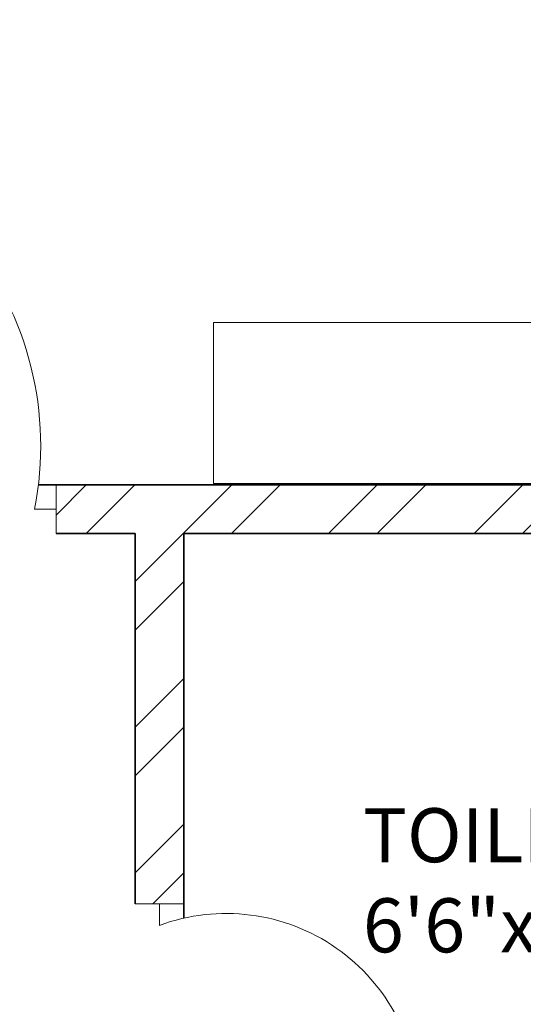
# Model space of a CAD drawing. Units: inches. Extents: x 2168 to 3056, y 1130 to 2629.
# Tile 35 of 42: x 2771 to 2818, y 2217 to 2308. Entities that reach past the tile are written whole.
import ezdxf

# ---------------------------------------------------------------- set-up
doc = ezdxf.new("R2010")
doc.units = ezdxf.units.IN
for name, color, linetype, lineweight in [('A-AREA-IDEN', 7, 'Continuous', 18), ('A-DOOR', 21, 'Continuous', 18), ('A-FLOR-CASE', 71, 'Continuous', 18), ('A-WALL', 7, 'Continuous', 35)]:
    doc.layers.add(name, color=color, linetype=linetype, lineweight=lineweight)
doc.layers.add('A-WALL-PATT', color=143, linetype='Continuous', lineweight=13, true_color=0x7aafdf)
doc.styles.get("Standard").update_dxf_attribs({"font": 'arial.ttf'})

# ---------------------------------------------------------------- blocks, each defined once
blk = doc.blocks.new('CUPBOARD-BEDROOM')
blk.add_lwpolyline([(0, 14.894), (70.359, 14.894), (70.359, 0), (0, 0)], close=True)

msp = doc.modelspace()

# ---------------------------------------------------------------- hatches: boundary and pattern name
at = {"layer": 'A-WALL-PATT'}
h = msp.add_hatch(dxfattribs=at)
h.set_pattern_fill('ANSI32', color=256)
h.paths.add_polyline_path([(2463.796, 2409.389), (2467.387, 2409.389), (2467.387, 2413.889), (2454.768, 2413.889), (2454.768, 2411.639), (2454.768, 2409.389), (2459.296, 2409.389), (2459.296, 2265.389), (2455.644, 2265.389), (2455.644, 2260.889), (2467.349, 2260.889), (2467.349, 2263.139), (2467.349, 2265.389), (2463.796, 2265.389)])
h.paths.add_polyline_path([(2431.596, 2413.889), (2409.647, 2413.889), (2409.647, 2409.389), (2431.596, 2409.389), (2431.596, 2411.639)])
h.paths.add_polyline_path([(2349.647, 2413.889), (2331.796, 2413.889), (2331.796, 2362.671), (2336.296, 2362.671), (2336.296, 2409.389), (2349.647, 2409.389), (2349.647, 2411.639)])
h.paths.add_polyline_path([(2634.149, 2411.639), (2634.149, 2413.889), (2562.293, 2413.889), (2562.293, 2409.389), (2595.796, 2409.389), (2595.796, 2280.309), (2595.826, 2280.309), (2595.826, 2265.389), (2499.91, 2265.389), (2499.91, 2260.889), (2550.796, 2260.889), (2550.796, 2117.308), (2555.296, 2117.308), (2555.296, 2168.08), (2571.93, 2168.08), (2571.93, 2176.889), (2559.796, 2176.889), (2559.796, 2256.389), (2640.796, 2256.389), (2640.796, 2176.889), (2626.428, 2176.889), (2626.428, 2168.08), (2645.296, 2168.08), (2645.296, 2116.637), (2649.796, 2116.637), (2649.796, 2260.889), (2691.251, 2260.889), (2691.251, 2263.139), (2691.251, 2265.389), (2670.655, 2265.389), (2670.655, 2265.365), (2600.296, 2265.365), (2600.296, 2280.258), (2600.296, 2409.389), (2634.149, 2409.389)])
h.paths.add_polyline_path([(2600.296, 2473.889), (2612.84, 2473.889), (2612.84, 2478.389), (2572.636, 2478.389), (2572.636, 2473.889), (2595.796, 2473.889), (2595.796, 2413.889), (2600.296, 2413.889)])
h.paths.add_polyline_path([(2535.796, 2473.889), (2548.636, 2473.889), (2548.636, 2478.389), (2531.396, 2478.389), (2531.396, 2413.889), (2521.6, 2413.889), (2521.6, 2409.389), (2539.239, 2409.389), (2539.239, 2411.639), (2539.239, 2413.889), (2535.796, 2413.889)])
h.paths.add_polyline_path([(2664.796, 2478.389), (2636.84, 2478.389), (2636.84, 2473.889), (2660.296, 2473.889), (2660.296, 2413.889), (2656.165, 2413.889), (2656.165, 2409.389), (2671.684, 2409.389), (2671.684, 2411.639), (2671.684, 2413.889), (2664.796, 2413.889)])
h.paths.add_polyline_path([(2705.942, 2413.889), (2695.684, 2413.889), (2695.684, 2409.389), (2705.942, 2409.389)])
h.paths.add_polyline_path([(2741.35, 2413.889), (2728.733, 2413.889), (2728.733, 2411.639), (2728.733, 2409.389), (2732.296, 2409.389), (2732.296, 2265.389), (2725.733, 2265.389), (2725.733, 2260.889), (2740.917, 2260.889), (2740.917, 2263.139), (2740.917, 2265.389), (2736.796, 2265.389), (2736.796, 2409.389), (2741.35, 2409.389)])
h.paths.add_polyline_path([(2785.655, 2413.889), (2764.546, 2413.889), (2764.486, 2409.389), (2785.655, 2409.389), (2785.655, 2411.639)])
h.paths.add_polyline_path([(2864.296, 2413.889), (2845.655, 2413.889), (2845.655, 2409.389), (2859.796, 2409.389), (2859.796, 2368.425), (2864.296, 2368.425)])
h.paths.add_polyline_path([(2864.296, 2308.425), (2862.046, 2308.425), (2859.796, 2308.425), (2859.796, 2265.389), (2774.483, 2265.389), (2774.483, 2263.139), (2774.483, 2260.889), (2781.796, 2260.889), (2781.796, 2226.654), (2786.296, 2226.654), (2786.296, 2260.889), (2859.796, 2260.889), (2859.796, 2241.352), (2864.296, 2241.352)])
h.paths.add_polyline_path([(2864.296, 2217.352), (2862.046, 2217.352), (2859.796, 2217.352), (2859.796, 2200.889), (2786.296, 2200.889), (2786.296, 2205.931), (2784.046, 2205.931), (2781.796, 2205.931), (2781.796, 2150.974), (2786.296, 2150.974), (2786.296, 2161.889), (2859.796, 2161.889), (2859.796, 2144.419), (2864.296, 2144.419)])
h.paths.add_polyline_path([(2859.796, 2196.389), (2859.796, 2166.389), (2786.296, 2166.389), (2786.296, 2196.389)], flags=16)
h.paths.add_polyline_path([(2864.296, 2108.419), (2862.046, 2108.419), (2859.796, 2108.419), (2859.796, 2080.889), (2786.296, 2080.889), (2786.296, 2111.993), (2781.796, 2111.993), (2781.796, 2080.889), (2649.796, 2080.889), (2649.796, 2086.036), (2647.546, 2086.036), (2645.296, 2086.036), (2645.296, 2071.739), (2649.796, 2071.739), (2649.796, 2076.389), (2781.796, 2076.389), (2781.796, 2041.792), (2786.296, 2041.792), (2786.296, 2076.389), (2859.796, 2076.389), (2859.796, 2058.577), (2864.296, 2058.577)])
h.paths.add_polyline_path([(2864.296, 2022.577), (2859.796, 2022.577), (2859.796, 1992.389), (2786.296, 1992.389), (2786.296, 1999.573), (2781.796, 1999.573), (2781.796, 1848.085), (2784.046, 1848.085), (2786.296, 1848.085), (2786.296, 1851.389), (2859.796, 1851.389), (2859.796, 1838.258), (2864.296, 1838.258)], flags=17)
h.paths.add_polyline_path([(2859.796, 1987.889), (2859.796, 1855.889), (2786.296, 1855.889), (2786.296, 1987.889)], flags=16)
h.paths.add_polyline_path([(2823.046, 1987.889), (2841.421, 1921.889), (2823.046, 1855.889)], flags=0)
h.paths.add_polyline_path([(2864.296, 1814.258), (2859.796, 1814.258), (2859.796, 1791.389), (2786.296, 1791.389), (2786.296, 1825.658), (2784.046, 1825.658), (2781.796, 1825.658), (2781.796, 1791.389), (2720.155, 1791.389), (2720.155, 1791.265), (2649.796, 1791.265), (2649.796, 1806.159), (2649.796, 2038.983), (2647.546, 2038.983), (2645.296, 2038.983), (2645.296, 1783.925), (2649.796, 1783.925), (2649.796, 1786.889), (2781.796, 1786.889), (2781.796, 1746.789), (2786.296, 1746.789), (2786.296, 1786.889), (2859.796, 1786.889), (2859.796, 1770.083), (2864.296, 1770.083)])
h.paths.add_polyline_path([(2864.296, 1734.083), (2862.046, 1734.083), (2859.796, 1734.083), (2859.796, 1705.889), (2786.296, 1705.889), (2786.296, 1714.166), (2781.796, 1714.166), (2781.796, 1660.527), (2786.296, 1660.527), (2786.296, 1666.889), (2859.796, 1666.889), (2859.796, 1648.342), (2864.296, 1648.342)])
h.paths.add_polyline_path([(2786.296, 1701.389), (2859.796, 1701.389), (2859.796, 1671.389), (2786.296, 1671.389)], flags=16)
h.paths.add_polyline_path([(2649.796, 1756.576), (2647.546, 1756.576), (2645.296, 1756.576), (2645.296, 1606.889), (2555.296, 1606.889), (2555.296, 1749.513), (2553.046, 1749.513), (2550.796, 1749.513), (2550.796, 1606.889), (2503.006, 1606.889), (2503.006, 1604.639), (2503.006, 1602.389), (2595.796, 1602.389), (2595.849, 1602.389), (2595.849, 1587.495), (2595.796, 1458.389), (2561.502, 1458.389), (2561.502, 1456.139), (2561.502, 1453.889), (2595.796, 1453.889), (2595.796, 1381.889), (2573.438, 1381.889), (2573.438, 1377.389), (2613.01, 1377.389), (2613.01, 1379.639), (2613.01, 1381.889), (2600.296, 1381.889), (2600.296, 1453.889), (2634.327, 1453.889), (2634.327, 1458.389), (2600.296, 1458.389), (2600.296, 1602.389), (2670.655, 1602.389), (2694.095, 1602.389), (2694.095, 1606.889), (2649.796, 1606.889)])
h.paths.add_polyline_path([(2736.796, 1602.389), (2741.562, 1602.389), (2741.562, 1606.889), (2726.203, 1606.889), (2726.203, 1604.639), (2726.203, 1602.389), (2732.296, 1602.389), (2732.296, 1458.389), (2727.899, 1458.389), (2727.899, 1453.889), (2740.821, 1453.889), (2740.821, 1456.139), (2740.821, 1458.389), (2736.796, 1458.389)])
h.paths.add_polyline_path([(2859.796, 1606.889), (2786.296, 1606.889), (2786.296, 1637.334), (2784.046, 1637.334), (2781.796, 1637.334), (2781.796, 1606.889), (2775.612, 1606.889), (2775.612, 1602.389), (2859.796, 1602.389)])
h.paths.add_polyline_path([(2864.296, 1624.342), (2862.046, 1624.342), (2859.796, 1624.342), (2859.796, 1570.39), (2864.296, 1570.39)])
h.paths.add_polyline_path([(2864.296, 1510.39), (2862.046, 1510.39), (2859.796, 1510.39), (2859.796, 1458.389), (2846.735, 1458.389), (2846.735, 1456.139), (2846.735, 1453.889), (2864.296, 1453.889)])
h.paths.add_polyline_path([(2786.735, 1458.389), (2765.444, 1458.389), (2765.444, 1453.889), (2786.735, 1453.889)])
h.paths.add_polyline_path([(2706.004, 1458.389), (2695.36, 1458.389), (2695.36, 1453.889), (2706.004, 1453.889), (2706.004, 1456.139)])
h.paths.add_polyline_path([(2671.36, 1456.139), (2671.36, 1458.389), (2655.986, 1458.389), (2655.986, 1456.139), (2655.986, 1453.889), (2660.296, 1453.889), (2660.296, 1381.889), (2637.01, 1381.889), (2637.01, 1377.389), (2664.796, 1377.389), (2664.796, 1453.889), (2671.36, 1453.889)], flags=17)
h.paths.add_polyline_path([(2539.829, 1458.389), (2520.237, 1458.389), (2520.237, 1453.889), (2531.296, 1453.889), (2531.296, 1377.389), (2546.449, 1377.389), (2546.449, 1379.639), (2546.449, 1381.889), (2535.796, 1381.889), (2535.796, 1453.889), (2539.829, 1453.889)], flags=17)
h.paths.add_polyline_path([(2496.237, 1458.389), (2489.13, 1458.389), (2489.13, 1453.889), (2496.237, 1453.889), (2496.237, 1456.139)])
h.paths.add_polyline_path([(2467.433, 1456.139), (2467.433, 1458.389), (2463.796, 1458.389), (2463.796, 1602.389), (2468.242, 1602.389), (2468.242, 1605.7), (2468.242, 1606.889), (2454.602, 1606.889), (2454.602, 1602.389), (2459.296, 1602.389), (2459.296, 1458.389), (2454.24, 1458.389), (2454.24, 1453.889), (2467.433, 1453.889)])
h.paths.add_polyline_path([(2431.601, 1456.139), (2431.601, 1458.389), (2411.386, 1458.389), (2411.386, 1453.889), (2431.601, 1453.889)])
h.paths.add_polyline_path([(2351.386, 1458.389), (2336.296, 1458.389), (2336.296, 1490.693), (2334.046, 1490.693), (2331.796, 1490.693), (2331.796, 1453.889), (2351.386, 1453.889), (2351.386, 1456.139)])
h.paths.add_polyline_path([(2336.296, 1629.705), (2331.796, 1629.705), (2331.796, 1552.317), (2336.296, 1552.317), (2336.296, 1602.389), (2406.655, 1602.389), (2423.472, 1602.389), (2423.472, 1606.889), (2418.796, 1606.889), (2418.796, 1643.678), (2416.546, 1643.678), (2414.296, 1643.678), (2414.296, 1606.889), (2336.296, 1606.889)])
h.paths.add_polyline_path([(2418.796, 1714.384), (2414.296, 1714.384), (2414.296, 1705.889), (2336.296, 1705.889), (2336.296, 1731.324), (2334.046, 1731.324), (2331.796, 1731.324), (2331.796, 1653.705), (2334.046, 1653.705), (2336.296, 1653.705), (2336.296, 1666.889), (2414.296, 1666.889), (2414.296, 1663.589), (2418.796, 1663.589)])
h.paths.add_polyline_path([(2336.296, 1701.389), (2414.296, 1701.389), (2414.296, 1671.389), (2336.296, 1671.389)], flags=16)
h.paths.add_polyline_path([(2555.296, 2040.059), (2550.796, 2040.059), (2550.796, 1791.389), (2550.561, 1791.205), (2480.202, 1791.205), (2418.796, 1791.389), (2418.796, 1825.448), (2416.546, 1825.448), (2414.296, 1825.448), (2414.296, 1791.389), (2336.296, 1791.389), (2336.296, 1806.409), (2331.796, 1806.409), (2331.796, 1767.324), (2336.296, 1767.324), (2336.296, 1786.889), (2414.296, 1786.889), (2414.296, 1745.457), (2418.796, 1745.457), (2418.796, 1786.889), (2550.796, 1786.889), (2550.796, 1783.011), (2555.296, 1783.011)])
h.paths.add_polyline_path([(2418.796, 1923.389), (2423.207, 1923.389), (2423.207, 1925.639), (2423.207, 1927.889), (2418.796, 1927.889), (2418.796, 2000.048), (2414.296, 2000.048), (2414.296, 1992.389), (2336.296, 1992.389), (2336.296, 1987.889), (2414.296, 1987.889), (2414.296, 1855.889), (2336.296, 1855.889), (2336.296, 1851.389), (2414.296, 1851.389), (2414.296, 1846.759), (2418.796, 1846.759)], flags=17)
h.paths.add_polyline_path([(2336.296, 2019.294), (2334.046, 2019.294), (2331.796, 2019.294), (2331.796, 1830.409), (2336.296, 1830.409)], flags=17)
h.paths.add_polyline_path([(2550.796, 1927.889), (2453.541, 1927.889), (2453.541, 1925.639), (2453.541, 1923.389), (2550.796, 1923.389)], flags=17)
h.paths.add_polyline_path([(2744.987, 1927.889), (2649.796, 1927.889), (2649.796, 1923.389), (2744.987, 1923.389), (2744.987, 1925.639)], flags=17)
h.paths.add_polyline_path([(2555.296, 2086.458), (2553.046, 2086.458), (2550.796, 2086.458), (2550.796, 2080.889), (2418.796, 2080.889), (2336.296, 2080.889), (2336.296, 2115.399), (2334.046, 2115.399), (2331.796, 2115.399), (2331.796, 2055.294), (2336.296, 2055.294), (2336.296, 2076.389), (2550.796, 2076.389), (2550.796, 2071.538), (2555.296, 2071.538)])
h.paths.add_polyline_path([(2418.796, 2121.389), (2414.296, 2121.389), (2414.296, 2080.889), (2418.796, 2080.889)])
h.paths.add_polyline_path([(2418.796, 2076.389), (2414.296, 2076.389), (2414.296, 2035.123), (2418.796, 2035.123)])
h.paths.add_polyline_path([(2422.868, 2263.139), (2422.868, 2265.389), (2406.655, 2265.389), (2406.655, 2265.359), (2336.296, 2265.359), (2336.296, 2280.252), (2336.296, 2302.671), (2334.046, 2302.671), (2331.796, 2302.671), (2331.796, 2246.853), (2336.296, 2246.853), (2336.296, 2260.889), (2414.296, 2260.889), (2414.296, 2223.996), (2418.796, 2223.996), (2418.796, 2260.889), (2422.868, 2260.889)])
h.paths.add_polyline_path([(2418.796, 2204.783), (2416.546, 2204.783), (2414.296, 2204.783), (2414.296, 2200.889), (2336.296, 2200.889), (2336.296, 2220.853), (2331.796, 2220.853), (2331.796, 2151.399), (2336.296, 2151.399), (2336.296, 2161.889), (2414.296, 2161.889), (2414.296, 2153.726), (2418.796, 2153.726)])
h.paths.add_polyline_path([(2414.296, 2196.389), (2414.296, 2166.389), (2336.296, 2166.389), (2336.296, 2196.389)], flags=16)
h.paths.add_polyline_path([(2375.296, 2181.389), (2336.296, 2166.389), (2336.296, 2196.389)], flags=0)
h.paths.add_polyline_path([(2809.595, 2172.34), (2838.804, 2172.34), (2838.804, 2190.997), (2809.595, 2190.997)], flags=8)
h.paths.add_polyline_path([(2849.75, 1919.585), (2849.75, 1952.672), (2831.093, 1952.672), (2831.093, 1919.585)], flags=8)
h.paths.add_polyline_path([(2808.875, 1901.967), (2808.875, 1937.85), (2790.149, 1937.85), (2790.149, 1901.967)], flags=8)
h.paths.add_polyline_path([(2806.285, 1671.896), (2835.493, 1671.896), (2835.493, 1690.553), (2806.285, 1690.553)], flags=8)
h.paths.add_polyline_path([(2353.186, 1676.549), (2382.395, 1676.549), (2382.395, 1695.207), (2353.186, 1695.207)], flags=8)
h.paths.add_polyline_path([(2360.083, 1832.308), (2389.241, 1832.308), (2389.241, 1850.966), (2360.083, 1850.966)], flags=25)
h.paths.add_polyline_path([(2354.822, 2167.823), (2384.031, 2167.823), (2384.031, 2186.481), (2354.822, 2186.481)], flags=8)

# ---------------------------------------------------------------- linework, layer by layer
at = {"layer": 'A-DOOR'}
for p, q in [((2774.483, 2260.889), (2774.483, 2265.389)), ((2774.483, 2265.389), (2774.483, 2265.389)), ((2774.483, 2265.389), (2774.483, 2263.139)), ((2774.483, 2263.139), (2772.483, 2263.139)), ((2781.796, 2226.654), (2781.796, 2226.654)), ((2781.796, 2226.654), (2786.296, 2226.654)), ((2786.296, 2226.654), (2782.948, 2226.654)), ((2784.046, 2226.654), (2784.046, 2224.654)), ((2786.296, 2226.654), (2786.296, 2226.654))]:
    msp.add_line(p, q, dxfattribs=at)
for centre, radius, start, end in [((2742.917, 2268.999), 30.14, 348.78965, 90), ((2790.22, 2207.931), 17.826, 360, 110.26488)]:
    msp.add_arc(centre, radius, start, end, dxfattribs=at)
at = {"layer": 'A-WALL'}
for p, q in [((2772.841, 2265.389), (2859.796, 2265.389)), ((2774.483, 2260.889), (2781.796, 2260.889)), ((2781.796, 2260.889), (2781.796, 2226.654)), ((2786.296, 2260.889), (2786.296, 2225.32)), ((2786.296, 2260.889), (2859.796, 2260.889))]:
    msp.add_line(p, q, dxfattribs=at)

# ---------------------------------------------------------------- block references
at = {"layer": 'A-FLOR-CASE'}
msp.add_blockref('CUPBOARD-BEDROOM', (2789.057, 2265.523), dxfattribs=at)

# ---------------------------------------------------------------- texts
at = {"layer": 'A-AREA-IDEN', "insert": (2802.88, 2235.492), "char_height": 5, "attachment_point": 1}
msp.add_mtext_dynamic_manual_height_columns('TOILET\\P6\'6"x5\'0"', width=169.35932, gutter_width=12.5, heights=[0], dxfattribs=at)

doc.saveas('drawing.dxf')
